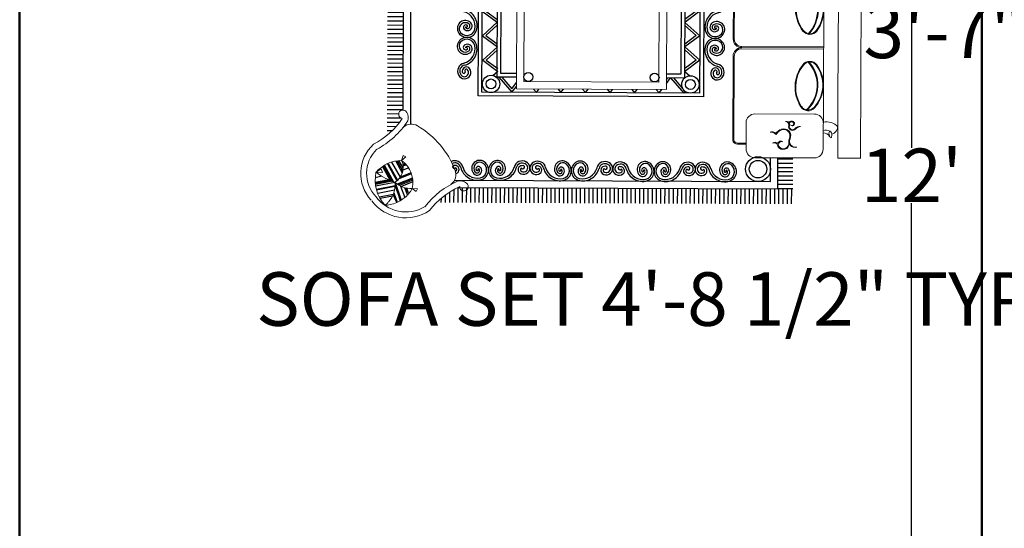
# Model space of a CAD drawing. Units: inches. Extents: x 147 to 1638, y 107 to 941.
# Tile 3 of 17: x 359 to 469, y 284 to 341. Entities that reach past the tile are written whole.
import ezdxf

# ---------------------------------------------------------------- set-up
doc = ezdxf.new("R2010")
doc.units = ezdxf.units.IN
doc.header["$MEASUREMENT"] = 0
for name, color, linetype, lineweight in [('A-ANNO-DIMS', 2, 'Continuous', 15), ('furniture', 50, 'Continuous', 18), ('wall', 7, 'Continuous', 60), ('walls', 7, 'Continuous', 50)]:
    doc.layers.add(name, color=color, linetype=linetype, lineweight=lineweight)
doc.layers.add('CARPET', color=40, linetype='Continuous')
doc.styles.get("Standard").update_dxf_attribs({"font": 'arial.ttf'})
doc.dimstyles.get("Standard").update_dxf_attribs({"dimtxt": 6, "dimasz": 3, "dimexe": 0.18, "dimexo": 0.0625, "dimgap": 0.09, "dimtad": 0, "dimtih": 1, "dimtoh": 1, "dimdec": 1, "dimzin": 0, "dimdsep": 46, "dimlunit": 3, "dimtxsty": 'Standard', "dimblk": 'ARCHTICK', "dimcen": 0.09, "dimadec": 0, "dimazin": 0, "dimtfac": 1, "dimtdec": 1, "dimtofl": 0, "dimtmove": 0, "dimatfit": 3, "dimfxl": 1, "dimtolj": 1, "dimtzin": 0, "dimarcsym": 0})

# ---------------------------------------------------------------- blocks, each defined once
blk = doc.blocks.new('_ArchTick')
at = {"color": 0, "linetype": 'ByBlock', "const_width": 0.15}
blk.add_lwpolyline([(-0.5, -0.5), (0.5, 0.5)], dxfattribs=at)
blk = doc.blocks.new('*D30')
at = {"layer": 'A-ANNO-DIMS', "color": 0, "lineweight": -2, "transparency": 16777216}
for p, q in [((460.3, 395.72), (458.86, 395.72)), ((459.04, 395.72), (459.04, 326.82)), ((459.04, 251.72), (459.04, 320.62)), ((460.3, 251.72), (458.86, 251.72))]:
    blk.add_line(p, q, dxfattribs=at)
at = {"layer": 'Defpoints', "color": 0, "lineweight": -2, "transparency": 16777216}
for p in [(460.36, 395.72), (459.04, 251.72), (460.36, 251.72)]:
    blk.add_point(p, dxfattribs=at)
at = {"layer": 'A-ANNO-DIMS', "color": 0, "lineweight": -2, "transparency": 16777216, "xscale": 3, "yscale": 3, "zscale": 3}
for p, rotation in [((459.04, 395.72), 90), ((459.04, 251.72), 270)]:
    blk.add_blockref('_ArchTick', p, dxfattribs=dict(at, rotation=rotation))
at = {"layer": 'A-ANNO-DIMS', "color": 0, "transparency": 16777216, "insert": (459.04, 323.72), "char_height": 6, "attachment_point": 5}
blk.add_mtext("\\A1;12'", dxfattribs=at)
blk = doc.blocks.new('X')
at = {"layer": 'furniture'}
for p, q in [((619.5149, -248.9209), (619.5149, -248.7654)), ((619.5149, -248.7654), (621.0036, -248.7654)), ((621.0036, -248.9205), (621.0036, -248.765)), ((619.5149, -248.9209), (619.7322, -248.9205)), ((619.7322, -248.9205), (620.6015, -248.9205)), ((621.0036, -248.9205), (620.6015, -248.9205)), ((619.5742, -249.0193), (619.752, -249.0193)), ((619.752, -249.0193), (620.6015, -249.0193)), ((620.2516, -249.5725), (620.2516, -249.0193)), ((620.259, -249.5725), (620.259, -249.0193)), ((620.259, -249.5725), (620.259, -249.0193)), ((620.2664, -249.5725), (620.2664, -249.0193)), ((620.9439, -249.0193), (620.6015, -249.0193)), ((619.5149, -249.0786), (619.5149, -249.4824)), ((619.8112, -249.4824), (619.8112, -249.0786)), ((620.7068, -249.4824), (620.7068, -249.0786)), ((621.0032, -249.4824), (621.0032, -249.0786)), ((619.5742, -249.5417), (619.752, -249.5417)), ((619.6049, -249.5417), (619.6049, -249.5987)), ((619.6124, -249.5417), (619.6124, -249.599)), ((620.9439, -249.5417), (620.7661, -249.5417)), ((620.9057, -249.5417), (620.9057, -249.599)), ((620.9131, -249.5417), (620.9131, -249.5987)), ((619.6334, -249.6243), (620.1998, -249.6243)), ((619.6334, -249.6317), (620.1998, -249.6317)), ((620.8846, -249.6243), (620.3183, -249.6243)), ((620.8846, -249.6317), (620.3183, -249.6317))]:
    blk.add_line(p, q, dxfattribs=at)
for centre, radius, start, end in [((619.7322, -248.9798), 0.0593, 90, 162.494), ((619.6556, -248.9979), 0.1044, 348.14652, 47.53007), ((620.8625, -248.9979), 0.1044, 132.46993, 191.85348), ((620.7859, -248.9798), 0.0593, 17.506, 90), ((619.635, -249.0188), 0.0496, 359.41182, 58.40348), ((619.6525, -249.0006), 0.0512, 338.60223, 29.59056), ((620.8656, -249.0006), 0.0512, 150.40944, 201.39777), ((620.8831, -249.0188), 0.0496, 121.59652, 180.58818), ((619.5742, -249.0786), 0.0593, 90, 180), ((619.752, -249.0786), 0.0593, 0, 90), ((620.007, -249.2904), 0.2333, 46.53167, 137.57273), ((620.007, -249.2476), 0.2283, 52.96969, 132.32477), ((620.007, -249.2476), 0.2234, 52.96969, 132.32477), ((620.5111, -249.2904), 0.2333, 42.42727, 133.46833), ((620.5111, -249.2476), 0.2283, 47.67523, 127.03031), ((620.5111, -249.2476), 0.2234, 47.67523, 127.03031), ((620.7661, -249.0786), 0.0593, 90, 180), ((620.9439, -249.0786), 0.0593, 0, 90), ((619.8932, -249.1226), 0.0593, 132.32477, 237.31292), ((620.007, -249.2904), 0.2283, 45.74065, 138.43075), ((619.8932, -249.1226), 0.0543, 132.32477, 237.31292), ((620.1088, -249.1127), 0.0543, 307.98154, 52.96969), ((620.1088, -249.1127), 0.0593, 307.98154, 52.96969), ((620.4092, -249.1127), 0.0593, 127.03031, 232.01846), ((620.5111, -249.2904), 0.2283, 41.56925, 134.25935), ((620.4092, -249.1127), 0.0543, 127.03031, 232.01846), ((620.6249, -249.1226), 0.0543, 302.68708, 47.67523), ((620.6249, -249.1226), 0.0593, 302.68708, 47.67523), ((619.6678, -249.1626), 0.0605, 312.99292, 349.19232), ((619.6905, -249.1804), 0.0373, 306.00619, 9.85592), ((619.994, -248.9656), 0.2459, 237.31292, 307.98154), ((619.994, -248.9656), 0.241, 237.31292, 307.98154), ((620.5241, -248.9656), 0.2459, 232.01846, 302.68708), ((620.5241, -248.9656), 0.241, 232.01846, 302.68708), ((620.8276, -249.1804), 0.0373, 170.14408, 233.99381), ((620.8503, -249.1626), 0.0605, 190.80768, 227.00708), ((619.6105, -249.2907), 0.0399, 81.34647, 244.80036), ((619.6138, -249.2892), 0.0378, 78.82007, 241.2356), ((619.6274, -249.2105), 0.0421, 161.95623, 295.85894), ((619.628, -249.2055), 0.0415, 168.85347, 291.99707), ((619.6641, -249.2863), 0.0471, 341.95623, 115.85894), ((619.6641, -249.2863), 0.0421, 341.95623, 115.85894), ((619.7278, -249.227), 0.0274, 132.99292, 265.5491), ((619.7278, -249.227), 0.0225, 132.99292, 262.0854), ((619.7361, -249.2716), 0.0251, 55.31815, 117.0875), ((619.7357, -249.2774), 0.0252, 3.68155, 113.53579), ((619.745, -249.2275), 0.014, 61.30612, 229.17278), ((619.7459, -249.2313), 0.0122, 73.4413, 214.10415), ((619.7406, -249.2356), 0.0182, 302.61304, 61.30612), ((619.7406, -249.2356), 0.0232, 306.28248, 61.30612), ((619.7361, -249.2716), 0.0251, 350.3606, 43.63947), ((620.7775, -249.2356), 0.0232, 118.69388, 233.71752), ((620.782, -249.2716), 0.0251, 136.36053, 189.6394), ((620.7824, -249.2774), 0.0252, 66.46421, 176.31845), ((620.7775, -249.2356), 0.0182, 118.69388, 237.38696), ((620.7731, -249.2275), 0.014, 310.82722, 118.69388), ((620.782, -249.2716), 0.0251, 62.9125, 124.68185), ((620.7722, -249.2313), 0.0122, 325.89585, 106.5587), ((620.7903, -249.227), 0.0274, 274.4509, 47.00708), ((620.7903, -249.227), 0.0225, 277.9146, 47.00708), ((620.854, -249.2863), 0.0471, 64.14106, 198.04377), ((620.854, -249.2863), 0.0421, 64.14106, 198.04377), ((620.8907, -249.2105), 0.0421, 244.14106, 18.04377), ((620.89, -249.2055), 0.0415, 248.00293, 11.14653), ((620.9043, -249.2892), 0.0378, 298.7644, 101.17993), ((620.9076, -249.2907), 0.0399, 295.19964, 98.65353), ((619.6028, -249.3007), 0.0227, 251.57956, 22.48814), ((619.6037, -249.3051), 0.024, 287.88795, 33.0148), ((619.6438, -249.2797), 0.0635, 295.85894, 341.95623), ((619.6438, -249.2797), 0.0684, 298.77648, 341.95623), ((620.8743, -249.2797), 0.0684, 198.04377, 241.22352), ((620.8743, -249.2797), 0.0635, 198.04377, 244.14106), ((620.9144, -249.3051), 0.024, 146.9852, 252.11205), ((620.9153, -249.3007), 0.0227, 157.51186, 288.42044), ((619.5921, -249.3513), 0.0246, 333.67342, 86.7751), ((619.5947, -249.3467), 0.0249, 321.27483, 48.99439), ((619.6335, -249.3751), 0.0539, 355.27866, 45.25264), ((619.6593, -249.3656), 0.0313, 333.5007, 56.06813), ((620.8588, -249.3656), 0.0313, 123.93187, 206.4993), ((620.8845, -249.3751), 0.0539, 134.74736, 184.72134), ((620.9233, -249.3467), 0.0249, 131.00561, 218.72517), ((620.926, -249.3513), 0.0246, 93.2249, 206.32658), ((619.5742, -249.4824), 0.0593, 180, 270), ((619.752, -249.4824), 0.0593, 270, 0), ((620.7661, -249.4824), 0.0593, 180, 270), ((620.9439, -249.4824), 0.0593, 270, 0), ((620.1998, -249.5725), 0.0593, 270, 0), ((620.1998, -249.5725), 0.0519, 270, 0), ((620.3183, -249.5725), 0.0593, 180, 270), ((620.3183, -249.5725), 0.0519, 180, 270), ((619.6387, -249.5984), 0.0338, 180.54468, 260.99104), ((619.6384, -249.5987), 0.0261, 179.37819, 258.97154), ((620.8796, -249.5987), 0.0261, 281.02846, 0.62181), ((620.8793, -249.5984), 0.0338, 279.00896, 359.45532)]:
    blk.add_arc(centre, radius, start, end, dxfattribs=at)
blk.add_ellipse((619.6743, -248.9709), major_axis=(-0.023, 0.0035), ratio=0.388107, start_param=3.141593, end_param=9.424778, dxfattribs=at)
at = {"layer": 'furniture', "extrusion": (0, 0, -1)}
blk.add_ellipse((620.8437, -248.9709), major_axis=(0.023, 0.0035), ratio=0.388107, start_param=3.141593, end_param=9.424778, dxfattribs=at)
blk = doc.blocks.new('sitting')
at = {"layer": 'CARPET'}
for p, q in [((0.3744, 0.8151), (0.3749, 0.9167)), ((0.403, 0.815), (0.4035, 0.9166)), ((0.4316, 0.8149), (0.432, 0.9165)), ((0.4602, 0.8148), (0.4606, 0.9164)), ((0.4887, 0.8147), (0.4892, 0.9163)), ((0.5173, 0.8145), (0.5178, 0.9161)), ((0.5459, 0.8144), (0.5463, 0.916)), ((0.5745, 0.8143), (0.5749, 0.9159)), ((0.603, 0.8142), (0.6035, 0.9158)), ((0.6316, 0.8141), (0.632, 0.9156)), ((0.6602, 0.8139), (0.6606, 0.9155)), ((0.6888, 0.8138), (0.6892, 0.9154)), ((2.1553, 0.8075), (2.1557, 0.9091)), ((2.1839, 0.8074), (2.1843, 0.909)), ((2.2125, 0.8073), (2.2129, 0.9089)), ((2.241, 0.8072), (2.2415, 0.9088)), ((2.2696, 0.8071), (2.27, 0.9087)), ((2.2982, 0.8069), (2.2986, 0.9085)), ((2.3268, 0.8068), (2.3272, 0.9084)), ((2.3553, 0.8067), (2.3558, 0.9083)), ((2.4602, 0.8713), (2.3589, 0.8717)), ((2.4603, 0.8998), (2.359, 0.9003)), ((0.3793, 0.8151), (0.3774, 0.3798)), ((0.6912, 0.81), (0.3793, 0.8151)), ((0.4301, 0.8149), (0.4301, 0.8143)), ((2.3583, 0.8067), (2.1476, 0.8076)), ((2.349, -1.3602), (2.3583, 0.8067)), ((2.4599, 0.8141), (2.3586, 0.8145)), ((2.46, 0.8427), (2.3588, 0.8431)), ((0.3789, 0.7373), (0.2773, 0.7377)), ((0.379, 0.7658), (0.2774, 0.7663)), ((0.3791, 0.7944), (0.2775, 0.7949)), ((0.3791, 0.7643), (0.3785, 0.7643)), ((0.4299, 0.7635), (0.4282, 0.3764)), ((0.6904, 0.7592), (0.4299, 0.7635)), ((2.3073, 0.7561), (2.1474, 0.7568)), ((2.2981, -1.3815), (2.3073, 0.7561)), ((2.4597, 0.757), (2.3584, 0.7574)), ((2.4598, 0.7855), (2.3585, 0.786)), ((0.3786, 0.6801), (0.277, 0.6806)), ((0.3788, 0.7087), (0.2772, 0.7091)), ((2.4593, 0.6712), (2.358, 0.6717)), ((2.4594, 0.6998), (2.3582, 0.7002)), ((2.4596, 0.7284), (2.3583, 0.7288)), ((0.3784, 0.623), (0.2768, 0.6234)), ((0.3785, 0.6515), (0.2769, 0.652)), ((2.4591, 0.6141), (2.3578, 0.6145)), ((2.4592, 0.6427), (2.3579, 0.6431)), ((0.378, 0.5372), (0.2764, 0.5377)), ((0.3782, 0.5658), (0.2766, 0.5663)), ((0.3783, 0.5944), (0.2767, 0.5948)), ((2.4588, 0.5569), (2.3576, 0.5574)), ((2.4589, 0.5855), (2.3577, 0.586)), ((0.3778, 0.4801), (0.2762, 0.4805)), ((0.3779, 0.5087), (0.2763, 0.5091)), ((2.4585, 0.4712), (2.3572, 0.4717)), ((2.4586, 0.4998), (2.3573, 0.5002)), ((2.4587, 0.5284), (2.3574, 0.5288)), ((0.3775, 0.4229), (0.2759, 0.4234)), ((0.3777, 0.4515), (0.2761, 0.452)), ((2.4582, 0.4141), (2.3569, 0.4145)), ((2.4583, 0.4426), (2.3571, 0.4431)), ((0.3774, 0.3944), (0.2758, 0.3948)), ((2.458, 0.3569), (2.3567, 0.3574)), ((2.4581, 0.3855), (2.3568, 0.3859)), ((1.065, 0.178), (1.1552, 0.2792)), ((1.1552, 0.2792), (1.2313, 0.1773)), ((1.2313, 0.1773), (1.3215, 0.2785)), ((1.3215, 0.2785), (1.3976, 0.1766)), ((1.3976, 0.1766), (1.4877, 0.2778)), ((1.4877, 0.2778), (1.5638, 0.1759)), ((2.4576, 0.2712), (2.3563, 0.2716)), ((2.4577, 0.2998), (2.3565, 0.3002)), ((2.4578, 0.3283), (2.3566, 0.3288)), ((1.0854, 0.1779), (1.1542, 0.2552)), ((1.1542, 0.2552), (1.2122, 0.1774)), ((1.2516, 0.1772), (1.3204, 0.2544)), ((1.3204, 0.2544), (1.3785, 0.1767)), ((1.4179, 0.1765), (1.4867, 0.2537)), ((1.4867, 0.2537), (1.5447, 0.176)), ((1.5638, 0.1759), (1.5928, 0.2111)), ((2.4574, 0.214), (2.3561, 0.2145)), ((2.4575, 0.2426), (2.3562, 0.2431)), ((1.0646, 0.0827), (0.9634, 0.1728)), ((1.0647, 0.103), (0.9951, 0.165)), ((1.6077, 0.0803), (1.7096, 0.1696)), ((1.6077, 0.1007), (1.6779, 0.1621)), ((1.7096, 0.1696), (1.6979, 0.1786)), ((2.4571, 0.1569), (2.3558, 0.1573)), ((2.4572, 0.1855), (2.356, 0.1859)), ((0.9627, 0.0066), (1.0646, 0.0827)), ((1.6441, 0.0527), (1.6077, 0.0803)), ((2.4567, 0.0712), (2.3555, 0.0716)), ((2.4569, 0.0997), (2.3556, 0.1002)), ((2.457, 0.1283), (2.3557, 0.1288)), ((1.0444, -0.0662), (0.9627, 0.0066)), ((0.9868, 0.0055), (1.0646, 0.0636)), ((1.0444, -0.0458), (0.9868, 0.0055)), ((1.6188, 0.0528), (1.6076, 0.0613)), ((1.6859, -0.0168), (1.7089, 0.0034)), ((1.7089, 0.0034), (1.6861, 0.0207)), ((2.4565, 0.014), (2.3552, 0.0145)), ((2.4566, 0.0426), (2.3554, 0.043)), ((2.4563, -0.0431), (2.355, -0.0427)), ((2.4564, -0.0146), (2.3551, -0.0141)), ((0.962, -0.1597), (1.0442, -0.0983)), ((0.9861, -0.1607), (1.0441, -0.1174)), ((2.4559, -0.1288), (2.3546, -0.1284)), ((2.456, -0.1003), (2.3547, -0.0998)), ((2.4561, -0.0717), (2.3549, -0.0713)), ((1.0436, -0.2324), (0.962, -0.1597)), ((1.0437, -0.2121), (0.9861, -0.1607)), ((1.6852, -0.183), (1.7082, -0.1629)), ((1.7082, -0.1629), (1.6854, -0.1455)), ((2.4557, -0.186), (2.3544, -0.1856)), ((2.4558, -0.1574), (2.3545, -0.157)), ((0.9613, -0.326), (1.0435, -0.2646)), ((2.4554, -0.2431), (2.3541, -0.2427)), ((2.4555, -0.2146), (2.3543, -0.2141)), ((1.0429, -0.3987), (0.9613, -0.326)), ((0.9854, -0.327), (1.0434, -0.2837)), ((1.043, -0.3784), (0.9854, -0.327)), ((1.6845, -0.3493), (1.7075, -0.3291)), ((1.7075, -0.3291), (1.6847, -0.3118)), ((2.455, -0.3289), (2.3538, -0.3284)), ((2.4552, -0.3003), (2.3539, -0.2999)), ((2.4553, -0.2717), (2.354, -0.2713)), ((0.3734, -0.5318), (0.374, -0.383)), ((0.4242, -0.5353), (0.4248, -0.38)), ((2.4548, -0.386), (2.3535, -0.3856)), ((2.4549, -0.3574), (2.3537, -0.357)), ((0.9606, -0.4922), (1.0428, -0.4308)), ((0.9847, -0.4933), (1.0427, -0.4499)), ((2.4546, -0.4432), (2.3533, -0.4427)), ((2.4547, -0.4146), (2.3534, -0.4142)), ((1.0422, -0.5649), (0.9606, -0.4922)), ((1.0423, -0.5446), (0.9847, -0.4933)), ((1.6838, -0.5155), (1.7068, -0.4954)), ((1.7068, -0.4954), (1.684, -0.478)), ((2.4542, -0.5289), (2.3529, -0.5285)), ((2.4543, -0.5003), (2.353, -0.4999)), ((2.4544, -0.4717), (2.3532, -0.4713)), ((0.9599, -0.6585), (1.0421, -0.5971)), ((2.4539, -0.586), (2.3527, -0.5856)), ((2.4541, -0.5575), (2.3528, -0.557)), ((1.0415, -0.7312), (0.9599, -0.6585)), ((0.984, -0.6595), (1.042, -0.6162)), ((1.0416, -0.7109), (0.984, -0.6595)), ((1.6831, -0.6818), (1.7061, -0.6617)), ((1.7061, -0.6617), (1.6833, -0.6443)), ((2.4537, -0.6432), (2.3524, -0.6428)), ((2.4538, -0.6146), (2.3526, -0.6142)), ((2.4533, -0.7289), (2.3521, -0.7285)), ((2.4535, -0.7003), (2.3522, -0.6999)), ((2.4536, -0.6718), (2.3523, -0.6713)), ((0.9592, -0.8247), (1.0414, -0.7634)), ((0.9832, -0.8258), (1.0413, -0.7824)), ((2.4531, -0.7861), (2.3518, -0.7856)), ((2.4532, -0.7575), (2.3519, -0.7571)), ((1.0408, -0.8975), (0.9592, -0.8247)), ((1.0409, -0.8771), (0.9832, -0.8258)), ((1.6824, -0.8481), (1.7054, -0.8279)), ((1.7054, -0.8279), (1.6825, -0.8106)), ((2.4528, -0.8432), (2.3516, -0.8428)), ((2.453, -0.8146), (2.3517, -0.8142)), ((0.9585, -0.991), (1.0407, -0.9296)), ((2.4525, -0.9289), (2.3512, -0.9285)), ((2.4526, -0.9004), (2.3513, -0.8999)), ((2.4527, -0.8718), (2.3515, -0.8714)), ((1.0597, -1.0812), (0.9585, -0.991)), ((0.9825, -0.992), (1.0406, -0.9487)), ((1.0598, -1.0608), (0.9825, -0.992)), ((1.6027, -1.0835), (1.7047, -0.9942)), ((1.6028, -1.0632), (1.6806, -0.995)), ((1.6806, -0.995), (1.6392, -0.9636)), ((1.7047, -0.9942), (1.6645, -0.9637)), ((2.4522, -0.9861), (2.351, -0.9857)), ((2.4524, -0.9575), (2.3511, -0.9571)), ((2.452, -1.0432), (2.3507, -1.0428)), ((2.4521, -1.0147), (2.3508, -1.0142)), ((1.0645, -1.0959), (1.1557, -1.1962)), ((1.0848, -1.0956), (1.1544, -1.1721)), ((1.1544, -1.1721), (1.2117, -1.0938)), ((1.1557, -1.1962), (1.2307, -1.0935)), ((1.2307, -1.0935), (1.3219, -1.1938)), ((1.2511, -1.0932), (1.3206, -1.1697)), ((1.3206, -1.1697), (1.3779, -1.0914)), ((1.3219, -1.1938), (1.397, -1.0911)), ((1.397, -1.0911), (1.4882, -1.1914)), ((1.4173, -1.0908), (1.4869, -1.1674)), ((1.4869, -1.1674), (1.5442, -1.089)), ((1.4882, -1.1914), (1.5632, -1.0887)), ((1.5632, -1.0887), (1.5926, -1.1237)), ((2.4516, -1.129), (2.3504, -1.1285)), ((2.4517, -1.1004), (2.3505, -1.1)), ((2.4519, -1.0718), (2.3506, -1.0714)), ((2.4514, -1.1861), (2.3501, -1.1857)), ((2.4515, -1.1575), (2.3502, -1.1571)), ((2.4511, -1.2433), (2.3499, -1.2428)), ((2.4513, -1.2147), (2.35, -1.2143)), ((0.3701, -1.3201), (0.2685, -1.3197)), ((0.3458, -1.2914), (0.2686, -1.2911)), ((0.3684, -1.73), (0.3702, -1.2947)), ((0.4194, -1.6792), (0.421, -1.2917)), ((2.4508, -1.329), (2.3495, -1.3286)), ((2.4509, -1.3004), (2.3496, -1.3)), ((2.451, -1.2718), (2.3498, -1.2714)), ((0.3699, -1.3773), (0.2683, -1.3768)), ((0.37, -1.3487), (0.2684, -1.3483)), ((2.4507, -1.3576), (2.3494, -1.3571)), ((2.4505, -1.3861), (2.3623, -1.3858)), ((0.3695, -1.463), (0.2679, -1.4626)), ((0.3696, -1.4344), (0.268, -1.434)), ((0.3697, -1.4058), (0.2681, -1.4054)), ((2.4504, -1.4147), (2.3793, -1.4144)), ((2.4503, -1.4433), (2.3989, -1.4431)), ((0.3693, -1.5201), (0.2677, -1.5197)), ((0.3694, -1.4916), (0.2678, -1.4911)), ((2.4502, -1.4719), (2.4215, -1.4717)), ((0.369, -1.5773), (0.2674, -1.5769)), ((0.3691, -1.5487), (0.2675, -1.5483)), ((0.3686, -1.663), (0.267, -1.6626)), ((0.3688, -1.6344), (0.2672, -1.634)), ((0.3689, -1.6059), (0.2673, -1.6054)), ((2.2845, -1.6663), (2.3262, -1.7708)), ((2.2896, -1.6655), (2.3296, -1.7657)), ((2.2995, -1.6644), (2.3358, -1.7553)), ((2.3112, -1.6637), (2.3424, -1.7417)), ((0.3684, -1.7202), (0.2668, -1.7197)), ((0.3685, -1.6916), (0.2669, -1.6912)), ((0.3684, -1.73), (1.8242, -1.7316)), ((0.3685, -1.6792), (0.3686, -1.6792)), ((0.3917, -1.8317), (0.3922, -1.7301)), ((0.4194, -1.6792), (1.9199, -1.6809)), ((0.4203, -1.8318), (0.4207, -1.7302)), ((0.4489, -1.8319), (0.4493, -1.7303)), ((0.4775, -1.832), (0.4779, -1.7304)), ((0.506, -1.8322), (0.5065, -1.7306)), ((0.5346, -1.8323), (0.535, -1.7307)), ((0.5632, -1.8324), (0.5636, -1.7308)), ((0.5917, -1.8325), (0.5922, -1.7309)), ((0.6203, -1.8327), (0.6208, -1.7311)), ((0.6489, -1.8328), (0.6493, -1.7312)), ((0.6775, -1.8329), (0.6779, -1.7313)), ((0.6775, -1.8329), (0.6779, -1.7313)), ((0.706, -1.833), (0.7065, -1.7314)), ((0.7346, -1.8331), (0.7351, -1.7315)), ((0.7632, -1.8333), (0.7636, -1.7317)), ((0.7918, -1.8334), (0.7922, -1.7318)), ((0.8203, -1.8335), (0.8208, -1.7319)), ((0.8489, -1.8336), (0.8494, -1.732)), ((0.8775, -1.8338), (0.8779, -1.7322)), ((0.9061, -1.8339), (0.9065, -1.7323)), ((0.9346, -1.834), (0.9351, -1.7324)), ((0.9632, -1.8341), (0.9637, -1.7325)), ((0.9632, -1.8341), (0.9637, -1.7325)), ((0.9918, -1.8342), (0.9922, -1.7326)), ((1.0204, -1.8344), (1.0208, -1.7328)), ((1.0489, -1.8345), (1.0494, -1.7329)), ((1.0775, -1.8346), (1.078, -1.733)), ((1.1061, -1.8347), (1.1065, -1.7331)), ((1.1347, -1.8349), (1.1351, -1.7333)), ((2.1669, -1.7607), (2.2209, -1.7306)), ((2.1682, -1.7716), (2.2377, -1.7329)), ((2.1869, -1.7158), (2.1934, -1.732)), ((2.1905, -1.7124), (2.1981, -1.7313)), ((2.1949, -1.7086), (2.2037, -1.7307)), ((2.2165, -1.6925), (2.2322, -1.7319)), ((2.2497, -1.6758), (2.2797, -1.7508)), ((2.2561, -1.6735), (2.2901, -1.7588)), ((2.3392, -1.7487), (2.4162, -1.7184)), ((2.3496, -1.7218), (2.4007, -1.7017)), ((2.3514, -1.7152), (2.3825, -1.7029)), ((2.353, -1.7075), (2.3836, -1.6955)), ((1.1632, -1.835), (1.1637, -1.7334)), ((1.1918, -1.8351), (1.1923, -1.7335)), ((1.2204, -1.8352), (1.2208, -1.7336)), ((1.249, -1.8353), (1.2494, -1.7337)), ((1.249, -1.8353), (1.2494, -1.7337)), ((1.2775, -1.8355), (1.278, -1.7339)), ((1.3061, -1.8356), (1.3066, -1.734)), ((1.3347, -1.8357), (1.3351, -1.7341)), ((1.3633, -1.8358), (1.3637, -1.7342)), ((1.3918, -1.8359), (1.3923, -1.7344)), ((1.4204, -1.8361), (1.4209, -1.7345)), ((1.449, -1.8362), (1.4494, -1.7346)), ((1.4776, -1.8363), (1.478, -1.7347)), ((1.5061, -1.8364), (1.5066, -1.7348)), ((1.5347, -1.8366), (1.5351, -1.735)), ((1.5347, -1.8366), (1.5351, -1.735)), ((1.5633, -1.8367), (1.5637, -1.7351)), ((1.5919, -1.8368), (1.5923, -1.7352)), ((1.6204, -1.8369), (1.6209, -1.7353)), ((1.649, -1.837), (1.6494, -1.7354)), ((1.6776, -1.8372), (1.678, -1.7356)), ((1.7062, -1.8373), (1.7066, -1.7357)), ((1.7347, -1.8374), (1.7352, -1.7358)), ((1.7633, -1.8375), (1.7637, -1.7359)), ((1.7919, -1.8377), (1.7923, -1.7361)), ((1.8205, -1.8378), (1.8209, -1.7362)), ((1.8205, -1.8378), (1.8209, -1.7362)), ((1.849, -1.8379), (1.8494, -1.7604)), ((1.8776, -1.838), (1.878, -1.7463)), ((1.9062, -1.8381), (1.9065, -1.7539)), ((1.9348, -1.8383), (1.935, -1.7772)), ((1.9348, -1.8383), (1.935, -1.7772)), ((2.1696, -1.7798), (2.2486, -1.7358)), ((2.1767, -1.8083), (2.2798, -1.7509)), ((2.1854, -1.8315), (2.2996, -1.7679)), ((2.1876, -1.8364), (2.3032, -1.7719)), ((2.1988, -1.8576), (2.3106, -1.7953)), ((2.3142, -1.7864), (2.3404, -1.9165)), ((2.3154, -1.7846), (2.4341, -1.7427)), ((2.3177, -1.7875), (2.4393, -1.7513)), ((2.3375, -1.7853), (2.3628, -1.9109)), ((2.3403, -1.7854), (2.3836, -1.7684)), ((2.3425, -1.7855), (2.3676, -1.9096)), ((2.3667, -1.7885), (2.3896, -1.9022)), ((2.3849, -1.7941), (2.4485, -1.7704)), ((2.3952, -1.797), (2.4141, -1.8911)), ((2.3975, -1.7979), (2.448, -1.7755)), ((1.9633, -1.8384), (1.9635, -1.8042)), ((2.2023, -1.8633), (2.3072, -1.8049)), ((2.2069, -1.8702), (2.3018, -1.8173)), ((2.297, -1.8281), (2.3153, -1.9188)), ((2.3011, -1.8189), (2.3211, -1.9184)), ((2.3067, -1.8053), (2.3293, -1.9175)), ((2.4068, -1.802), (2.4237, -1.8859)), ((2.2731, -1.8735), (2.2823, -1.919))]:
    blk.add_line(p, q, dxfattribs=at)
for points in [[(0.9321, -1.2188), (0.9386, 0.3056), (1.7356, 0.3022), (1.7291, -1.2222)], [(0.9576, -1.1935), (0.9639, 0.2801), (1.7101, 0.2769), (1.7038, -1.1967)]]:
    blk.add_lwpolyline(points, close=True, dxfattribs=at)
for points in [[(1.0645, 0.0551), (1.065, 0.178), (1.6081, 0.1757), (1.6075, 0.0528)], [(1.0899, 0.055), (1.0903, 0.1525), (1.5826, 0.1504), (1.5821, 0.0529)], [(1.6032, -0.9634), (1.6026, -1.0947), (1.0596, -1.0923), (1.0602, -0.9611)], [(1.5778, -0.9633), (1.5774, -1.0692), (1.0851, -1.0671), (1.0856, -0.9612)]]:
    blk.add_lwpolyline(points, dxfattribs=at)
for centre, radius in [((0.5147, 0.6796), 0.0843), ((0.5147, 0.6796), 0.0589), ((2.2246, 0.6725), 0.0843), ((2.2246, 0.6725), 0.0589), ((1.022, 0.2174), 0.0589), ((1.6516, 0.2147), 0.0589), ((1.022, 0.2174), 0.0335), ((1.6516, 0.2147), 0.0335), ((1.1262, -0.0259), 0.0301), ((1.6047, -0.028), 0.0301), ((1.1225, -0.881), 0.0301), ((1.601, -0.883), 0.0301), ((1.0184, -1.1325), 0.0589), ((1.0184, -1.1325), 0.0335), ((1.6479, -1.1352), 0.0589), ((1.6479, -1.1352), 0.0335), ((0.505, -1.5948), 0.0843), ((0.505, -1.5948), 0.0589)]:
    blk.add_circle(centre, radius, dxfattribs=at)
for centre, radius, start, end in [((0.497, 0.4669), 0.067, 33.92326, 162.74749), ((0.5416, 0.4551), 0.1132, 163.72753, 224.16333), ((0.5428, 0.4571), 0.1008, 166.99629, 238.96019), ((0.4977, 0.4665), 0.0548, 20.90664, 165.92882), ((0.4936, 0.4564), 0.0315, 41.04313, 239.89648), ((0.4936, 0.4564), 0.0169, 41.04313, 239.89648), ((0.5086, 0.4733), 0.0538, 235.07981, 35.18035), ((0.5086, 0.4759), 0.0415, 235.36127, 14.07703), ((0.5048, 0.4662), 0.0166, 231.08782, 41.04313), ((0.5048, 0.4662), 0.00198, 231.08782, 41.04313), ((2.2298, 0.466), 0.0538, 144.33076, 304.4313), ((2.2413, 0.4595), 0.067, 16.76363, 145.58785), ((2.2297, 0.4686), 0.0415, 165.43408, 304.14985), ((2.2406, 0.459), 0.0548, 13.58229, 158.60447), ((2.2335, 0.4588), 0.0166, 138.46799, 308.4233), ((2.1954, 0.45), 0.1008, 284.1961, 12.51483), ((2.2447, 0.449), 0.0315, 299.61464, 138.46799), ((2.1966, 0.448), 0.1132, 284.45049, 15.78359), ((0.5005, 0.4578), 0.00755, 65.8585, 269.29351), ((1.1039, 0.3982), 0.0436, 112.88129, 307.21618), ((1.1031, 0.3985), 0.0284, 110.32478, 311.53076), ((1.1129, 0.3899), 0.055, 11.99051, 119.18067), ((1.1129, 0.3899), 0.0404, 11.99051, 119.18067), ((1.1077, 0.403), 0.011, 65.50738, 327.11735), ((1.1131, 0.3853), 0.0277, 308.26022, 91.73038), ((1.264, 0.4277), 0.1008, 194.1961, 282.51483), ((1.2799, 0.3933), 0.0538, 54.33076, 214.4313), ((1.2629, 0.3785), 0.0315, 209.61464, 48.46799), ((1.2825, 0.3934), 0.0415, 75.43408, 214.14985), ((1.2728, 0.3896), 0.0166, 48.46799, 218.4233), ((1.273, 0.3825), 0.0548, 283.58229, 68.60447), ((1.2734, 0.3818), 0.067, 286.76363, 55.58785), ((1.4074, 0.3811), 0.067, 123.92326, 252.74749), ((1.4078, 0.3819), 0.0548, 110.90664, 255.92882), ((1.401, 0.3927), 0.0538, 325.07981, 125.18035), ((1.4179, 0.3777), 0.0315, 131.04313, 329.89648), ((1.3984, 0.3928), 0.0415, 325.36127, 104.07703), ((1.4172, 0.4269), 0.1008, 256.99629, 345.31502), ((1.4081, 0.389), 0.0166, 321.08782, 131.04313), ((1.5679, 0.3879), 0.055, 60.33045, 167.52061), ((1.5679, 0.3879), 0.0404, 60.33045, 167.52061), ((1.5677, 0.3833), 0.0277, 87.78073, 231.2509), ((1.577, 0.3961), 0.0436, 232.29494, 66.62983), ((1.5778, 0.3964), 0.0284, 227.98036, 69.18634), ((1.5733, 0.4009), 0.011, 212.39376, 114.00374), ((2.2335, 0.4588), 0.00198, 138.46799, 308.4233), ((2.2447, 0.449), 0.0169, 299.61464, 138.46799), ((2.2377, 0.4504), 0.00755, 270.2176, 113.65261), ((1.1133, 0.3856), 0.012, 316.00944, 72.44807), ((1.262, 0.4266), 0.1132, 194.45049, 285.78359), ((1.2629, 0.3785), 0.0169, 209.61464, 48.46799), ((1.2643, 0.3854), 0.00755, 180.2176, 23.65261), ((1.2728, 0.3896), 0.00198, 48.46799, 218.4233), ((1.4192, 0.4258), 0.1132, 253.72753, 345.06062), ((1.4179, 0.3777), 0.0169, 131.04313, 329.89648), ((1.4081, 0.389), 0.00198, 321.08782, 131.04313), ((1.4165, 0.3846), 0.00755, 155.8585, 359.29351), ((1.5675, 0.3835), 0.012, 107.06305, 223.50168), ((2.2332, 0.299), 0.055, 101.99051, 209.18067), ((2.2332, 0.299), 0.0404, 101.99051, 209.18067), ((2.2249, 0.29), 0.0436, 202.88129, 37.21618), ((2.2246, 0.2892), 0.0284, 200.32478, 41.53076), ((2.2201, 0.2937), 0.011, 155.50738, 57.11735), ((2.2378, 0.2991), 0.0277, 38.26022, 181.73038), ((2.2376, 0.2994), 0.012, 46.00944, 162.44807), ((2.2327, 0.1959), 0.055, 150.33045, 257.52061), ((2.2245, 0.205), 0.0436, 322.29494, 156.62983), ((2.2327, 0.1959), 0.0404, 150.33045, 257.52061), ((2.2243, 0.2058), 0.0284, 317.98036, 159.18634), ((2.2197, 0.2012), 0.011, 302.39376, 204.00374), ((2.2374, 0.1957), 0.0277, 177.78073, 321.2509), ((2.1937, 0.0451), 0.1008, 346.99629, 75.31502), ((2.1948, 0.0472), 0.1132, 343.72753, 75.06062), ((2.2371, 0.1955), 0.012, 197.06305, 313.50168), ((2.2279, 0.0289), 0.0538, 55.07981, 215.18035), ((2.2278, 0.0263), 0.0415, 55.36127, 194.07703), ((2.2429, 0.0458), 0.0315, 221.04313, 59.89648), ((2.2395, 0.0353), 0.067, 213.92326, 342.74749), ((2.2388, 0.0358), 0.0548, 200.90664, 345.92882), ((2.2317, 0.036), 0.0166, 51.08782, 221.04313), ((2.2317, 0.036), 0.00198, 51.08782, 221.04313), ((2.2429, 0.0458), 0.0169, 221.04313, 59.89648), ((2.236, 0.0445), 0.00755, 245.8585, 89.29351), ((2.2275, -0.0922), 0.0538, 144.33076, 304.4313), ((2.239, -0.0986), 0.067, 16.76363, 145.58785), ((2.2383, -0.0991), 0.0548, 13.58229, 158.60447), ((2.2274, -0.0895), 0.0415, 165.43408, 304.14985), ((2.2312, -0.0993), 0.0166, 138.46799, 308.4233), ((2.1931, -0.1081), 0.1008, 284.1961, 12.51483), ((2.2424, -0.1091), 0.0315, 299.61464, 138.46799), ((2.1942, -0.1101), 0.1132, 284.45049, 15.78359), ((2.2312, -0.0993), 0.00198, 138.46799, 308.4233), ((2.2424, -0.1091), 0.0169, 299.61464, 138.46799), ((2.2354, -0.1077), 0.00755, 270.2176, 113.65261), ((2.2309, -0.2591), 0.055, 101.99051, 209.18067), ((2.2226, -0.2681), 0.0436, 202.88129, 37.21618), ((2.2309, -0.2591), 0.0404, 101.99051, 209.18067), ((2.2223, -0.2689), 0.0284, 200.32478, 41.53076), ((2.2178, -0.2644), 0.011, 155.50738, 57.11735), ((2.2355, -0.259), 0.0277, 38.26022, 181.73038), ((2.2352, -0.2587), 0.012, 46.00944, 162.44807), ((2.22, -0.3553), 0.0436, 322.29494, 156.62983), ((2.2197, -0.3545), 0.0284, 317.98036, 159.18634), ((2.2282, -0.3643), 0.055, 150.33045, 257.52061), ((2.2282, -0.3643), 0.0404, 150.33045, 257.52061), ((2.2152, -0.359), 0.011, 302.39376, 204.00374), ((2.2328, -0.3646), 0.0277, 177.78073, 321.2509), ((2.2326, -0.3648), 0.012, 197.06305, 313.50168), ((2.1892, -0.5151), 0.1008, 346.99629, 75.31502), ((2.1903, -0.5131), 0.1132, 343.72753, 75.06062), ((2.2234, -0.5313), 0.0538, 55.07981, 215.18035), ((2.2233, -0.5339), 0.0415, 55.36127, 194.07703), ((2.2276, -0.5255), 0.0166, 51.08782, 221.04313), ((2.2384, -0.5144), 0.0315, 221.04313, 59.89648), ((2.2384, -0.5144), 0.0169, 221.04313, 59.89648), ((2.2276, -0.5255), 0.00198, 51.08782, 221.04313), ((2.232, -0.5171), 0.00755, 245.8585, 89.29351), ((2.2345, -0.6588), 0.067, 16.76363, 145.58785), ((2.235, -0.5249), 0.067, 213.92326, 342.74749), ((2.2342, -0.5244), 0.0548, 200.90664, 345.92882), ((2.2229, -0.6524), 0.0538, 144.33076, 304.4313), ((2.2229, -0.6498), 0.0415, 165.43408, 304.14985), ((2.2337, -0.6593), 0.0548, 13.58229, 158.60447), ((2.2271, -0.6608), 0.0166, 138.46799, 308.4233), ((2.1886, -0.6683), 0.1008, 284.1961, 12.51483), ((2.2378, -0.6694), 0.0315, 299.61464, 138.46799), ((2.1897, -0.6703), 0.1132, 284.45049, 15.78359), ((2.2378, -0.6694), 0.0169, 299.61464, 138.46799), ((2.2271, -0.6608), 0.00198, 138.46799, 308.4233), ((2.2314, -0.6693), 0.00755, 270.2176, 113.65261), ((2.2263, -0.8194), 0.055, 101.99051, 209.18067), ((2.2263, -0.8194), 0.0404, 101.99051, 209.18067), ((2.2309, -0.8192), 0.0277, 38.26022, 181.73038), ((2.218, -0.8284), 0.0436, 202.88129, 37.21618), ((2.2177, -0.8292), 0.0284, 200.32478, 41.53076), ((2.2132, -0.8246), 0.011, 155.50738, 57.11735), ((2.2307, -0.819), 0.012, 46.00944, 162.44807), ((2.2242, -0.9246), 0.055, 150.33045, 257.52061), ((2.216, -0.9155), 0.0436, 322.29494, 156.62983), ((2.2242, -0.9246), 0.0404, 150.33045, 257.52061), ((2.2157, -0.9147), 0.0284, 317.98036, 159.18634), ((2.2112, -0.9192), 0.011, 302.39376, 204.00374), ((2.2288, -0.9248), 0.0277, 177.78073, 321.2509), ((2.2286, -0.925), 0.012, 197.06305, 313.50168), ((2.1852, -1.0753), 0.1008, 346.99629, 75.31502), ((2.1863, -1.0733), 0.1132, 343.72753, 75.06062), ((2.2194, -1.0915), 0.0538, 55.07981, 215.18035), ((2.2193, -1.0941), 0.0415, 55.36127, 194.07703), ((2.2344, -1.0746), 0.0315, 221.04313, 59.89648), ((2.2344, -1.0746), 0.0169, 221.04313, 59.89648), ((2.231, -1.0852), 0.067, 213.92326, 342.74749), ((2.2302, -1.0847), 0.0548, 200.90664, 345.92882), ((2.2231, -1.0844), 0.0166, 51.08782, 221.04313), ((2.2231, -1.0844), 0.00198, 51.08782, 221.04313), ((2.2275, -1.076), 0.00755, 245.8585, 89.29351), ((2.2189, -1.2126), 0.0538, 144.33076, 304.4313), ((2.2305, -1.2191), 0.067, 16.76363, 145.58785), ((2.2189, -1.21), 0.0415, 165.43408, 304.14985), ((2.2297, -1.2195), 0.0548, 13.58229, 158.60447), ((2.2338, -1.2296), 0.0315, 299.61464, 138.46799), ((2.1857, -1.2305), 0.1132, 284.45049, 15.78359), ((1.2544, -1.3426), 0.1132, 73.72753, 165.06062), ((1.2564, -1.3437), 0.1008, 76.99629, 165.31502), ((1.2558, -1.2945), 0.0315, 311.04313, 149.89648), ((1.2658, -1.2986), 0.0548, 290.90664, 75.92882), ((1.2663, -1.2979), 0.067, 303.92326, 72.74749), ((1.4002, -1.2984), 0.067, 106.76363, 235.58785), ((1.4007, -1.2991), 0.0548, 103.58229, 248.60447), ((1.4107, -1.295), 0.0315, 29.61464, 228.46799), ((1.4117, -1.3432), 0.1132, 14.45049, 105.78359), ((1.4096, -1.3443), 0.1008, 14.1961, 102.51483), ((2.2231, -1.221), 0.0166, 138.46799, 308.4233), ((2.1846, -1.2285), 0.1008, 284.1961, 12.51483), ((2.2338, -1.2296), 0.0169, 299.61464, 138.46799), ((2.2231, -1.221), 0.00198, 138.46799, 308.4233), ((2.2274, -1.2295), 0.00755, 270.2176, 113.65261), ((0.5381, -1.2235), 0.1132, 217.11392, 255.06062), ((0.5393, -1.2215), 0.1008, 221.67675, 255.31502), ((0.5002, -1.3723), 0.0404, 330.33045, 77.52061), ((0.5002, -1.3723), 0.055, 330.33045, 77.52061), ((1.0966, -1.3129), 0.0436, 52.29494, 246.62983), ((1.0958, -1.3131), 0.0284, 47.98036, 249.18634), ((1.1057, -1.3047), 0.055, 240.33045, 347.52061), ((1.1057, -1.3047), 0.0404, 240.33045, 347.52061), ((1.1003, -1.3177), 0.011, 32.39376, 294.00374), ((1.1059, -1.3), 0.0277, 267.78073, 51.2509), ((1.1061, -1.3003), 0.012, 287.06305, 43.50168), ((1.2726, -1.3095), 0.0538, 145.07981, 305.18035), ((1.2753, -1.3096), 0.0415, 145.36127, 284.07703), ((1.2558, -1.2945), 0.0169, 311.04313, 149.89648), ((1.2656, -1.3057), 0.0166, 141.08782, 311.04313), ((1.2571, -1.3014), 0.00755, 335.8585, 179.29351), ((1.2656, -1.3057), 0.00198, 141.08782, 311.04313), ((1.3937, -1.3099), 0.0538, 234.33076, 34.4313), ((1.3911, -1.31), 0.0415, 255.43408, 34.14985), ((1.4008, -1.3062), 0.0166, 228.46799, 38.4233), ((1.4107, -1.295), 0.0169, 29.61464, 228.46799), ((1.4008, -1.3062), 0.00198, 228.46799, 38.4233), ((1.4093, -1.302), 0.00755, 0.2176, 203.65261), ((1.5607, -1.3065), 0.055, 191.99051, 299.18067), ((1.5607, -1.3065), 0.0404, 191.99051, 299.18067), ((1.5605, -1.3019), 0.0277, 128.26022, 271.73038), ((1.5697, -1.3148), 0.0436, 292.88129, 127.21618), ((1.5603, -1.3022), 0.012, 136.00944, 252.44807), ((1.5705, -1.3151), 0.0284, 290.32478, 131.53076), ((1.5659, -1.3196), 0.011, 245.50738, 147.11735), ((2.2223, -1.3796), 0.055, 101.99051, 209.18067), ((0.5085, -1.3813), 0.0436, 142.29494, 336.62983), ((0.4956, -1.372), 0.0277, 357.78073, 141.2509), ((0.5087, -1.3821), 0.0284, 137.98036, 339.18634), ((0.4959, -1.3718), 0.012, 17.06305, 133.50168), ((0.5133, -1.3776), 0.011, 122.39376, 24.00374), ((2.2223, -1.3796), 0.0404, 101.99051, 209.18067), ((2.2092, -1.3848), 0.011, 155.50738, 57.11735), ((2.2269, -1.3794), 0.0277, 38.26022, 181.73038), ((2.2267, -1.3792), 0.012, 46.00944, 162.44807), ((2.2137, -1.3894), 0.0284, 26.97547, 41.53076), ((2.214, -1.3886), 0.0436, 20.31739, 37.21618)]:
    blk.add_arc(centre, radius, start, end, dxfattribs=at)
at = {"layer": 'furniture'}
for p, q in [((-0.0014, -0.3337), (0.0014, 0.3337)), ((0.0011, -0.3483), (0.0041, 0.3483)), ((0.1243, -0.3679), (0.1274, 0.3668)), ((0.1263, -0.3665), (0.1294, 0.3654)), ((0.4025, 0.3765), (0.4672, 0.3762)), ((0.473, 0.3708), (0.6194, 0.3702)), ((0.4789, 0.3601), (0.6193, 0.3595)), ((0.4802, 0.3548), (0.6193, 0.3542)), ((0.129, 0.2827), (0.3801, 0.2816)), ((0.1292, 0.319), (0.3914, 0.3179)), ((0.4057, 0.326), (0.4705, 0.3258)), ((0.6537, -0.3223), (0.6564, 0.3168)), ((0.659, -0.3224), (0.6618, 0.3167)), ((0.6697, -0.3224), (0.6724, 0.3167)), ((1.0405, -0.961), (1.0449, 0.0552)), ((1.0449, 0.0552), (1.6862, 0.0525)), ((1.0916, -0.9104), (1.0955, 0.0042)), ((1.0955, 0.0042), (1.6352, 0.0019)), ((1.6352, 0.0019), (1.6313, -0.9127)), ((1.6862, 0.0525), (1.6819, -0.9637)), ((0.1265, -0.3201), (0.3887, -0.3212)), ((0.1266, -0.2838), (0.3777, -0.2849)), ((0.4029, -0.3295), (0.4677, -0.3298)), ((0.3992, -0.3799), (0.464, -0.3802)), ((0.4698, -0.3748), (0.6162, -0.3754)), ((0.4758, -0.3642), (0.6162, -0.3648)), ((0.4772, -0.3589), (0.6163, -0.3595)), ((-0.0025, -0.578), (-0.0053, -1.2453)), ((0.0002, -0.5633), (-0.0028, -1.26)), ((0.1235, -0.5449), (0.1204, -1.2795)), ((0.1255, -0.5462), (0.1224, -1.2782)), ((0.1253, -0.5926), (0.3875, -0.5938)), ((0.3986, -0.5351), (0.4633, -0.5354)), ((0.4019, -0.5856), (0.4666, -0.5859)), ((0.4691, -0.5409), (0.6155, -0.5415)), ((0.475, -0.5515), (0.6154, -0.5521)), ((0.4763, -0.5569), (0.6154, -0.5575)), ((0.6525, -0.5949), (0.6498, -1.234)), ((0.6579, -0.5949), (0.6551, -1.234)), ((0.6685, -0.595), (0.6658, -1.2341)), ((0.1251, -0.6289), (0.3763, -0.63)), ((1.6313, -0.9127), (1.0916, -0.9104)), ((1.6819, -0.9637), (1.0405, -0.961)), ((0.1227, -1.1955), (0.3738, -1.1965)), ((0.1226, -1.2317), (0.3848, -1.2329)), ((0.3991, -1.2411), (0.4638, -1.2414)), ((0.3953, -1.2916), (0.4601, -1.2918)), ((0.4659, -1.2865), (0.6123, -1.2871)), ((0.4719, -1.2758), (0.6124, -1.2764)), ((0.4733, -1.2705), (0.6124, -1.2711)), ((2.328, -1.4065), (2.3242, -1.4019)), ((2.3579, -1.6334), (2.3559, -1.6681)), ((2.3559, -1.6681), (2.3749, -1.643)), ((2.3749, -1.643), (2.3579, -1.6334)), ((1.9388, -1.7267), (1.9426, -1.7313)), ((2.1403, -1.7119), (2.1319, -1.7302)), ((2.1319, -1.7302), (2.1658, -1.7403)), ((2.1658, -1.7403), (2.1403, -1.7119)), ((2.2476, -1.8704), (2.2234, -1.878)), ((2.2234, -1.878), (2.2459, -1.914)), ((2.2459, -1.914), (2.2476, -1.8704))]:
    blk.add_line(p, q, dxfattribs=at)
for centre, radius, start, end in [((0.044, 0.3335), 0.0426, 119.85526, 179.75556), ((0.0722, 0.2845), 0.0991, 54.75501, 119.85526), ((0.1554, 2.0606), 1.6953, 269.12157, 278.01225), ((0.3827, 0.3499), 0.0332, 285.20211, 74.309), ((0.3862, 0.3499), 0.0332, 314.00797, 53.43036), ((0.4039, 0.3498), 0.0332, 314.00797, 53.43036), ((0.4192, 0.3497), 0.0332, 314.00797, 53.43036), ((0.4322, 0.3497), 0.0332, 314.00797, 53.43036), ((0.4416, 0.3496), 0.0332, 314.00797, 53.43036), ((0.4451, 0.3496), 0.0332, 314.00797, 53.43036), ((0.4475, 0.3496), 0.0332, 314.00797, 53.43036), ((0.6192, 0.3169), 0.0426, 359.75556, 89.75556), ((0.6192, 0.3169), 0.0373, 359.75556, 89.75556), ((0.6192, 0.3169), 0.0533, 359.75556, 89.75556), ((0.4606, 0.2765), 0.0806, 149.12023, 176.36211), ((0.4582, -0.2804), 0.0806, 183.14901, 210.39088), ((0.3797, -0.3531), 0.0332, 285.20211, 74.309), ((0.3832, -0.3531), 0.0332, 306.08075, 45.50314), ((0.4009, -0.3532), 0.0332, 306.08075, 45.50314), ((0.4162, -0.3533), 0.0332, 306.08075, 45.50314), ((0.4292, -0.3533), 0.0332, 306.08075, 45.50314), ((0.4386, -0.3534), 0.0332, 306.08075, 45.50314), ((0.4421, -0.3534), 0.0332, 306.08075, 45.50314), ((0.4445, -0.3534), 0.0332, 306.08075, 45.50314), ((0.6164, -0.3222), 0.0533, 269.75556, 359.75556), ((0.6164, -0.3222), 0.0533, 269.75556, 359.75556), ((0.6164, -0.3222), 0.0426, 269.75556, 359.75556), ((0.6164, -0.3222), 0.0373, 269.75556, 359.75556), ((0.0412, -0.3339), 0.0426, 179.75556, 239.65586), ((0.0697, -0.2851), 0.0991, 239.65586, 304.7561), ((0.1378, -2.0618), 1.6953, 81.49887, 90.38955), ((0.0683, -0.6272), 0.0991, 54.75501, 119.85526), ((0.1515, 1.1489), 1.6953, 269.12157, 278.01225), ((0.3788, -0.5618), 0.0332, 285.20211, 74.309), ((0.0401, -0.5781), 0.0426, 119.85526, 179.75556), ((0.4567, -0.6351), 0.0806, 149.12023, 176.36211), ((0.3823, -0.5618), 0.0332, 314.00797, 53.43036), ((0.4, -0.5619), 0.0332, 314.00797, 53.43036), ((0.4153, -0.5619), 0.0332, 314.00797, 53.43036), ((0.4283, -0.562), 0.0332, 314.00797, 53.43036), ((0.4377, -0.562), 0.0332, 314.00797, 53.43036), ((0.4412, -0.562), 0.0332, 314.00797, 53.43036), ((0.4436, -0.5621), 0.0332, 314.00797, 53.43036), ((0.6153, -0.5947), 0.0426, 359.75556, 89.75556), ((0.6153, -0.5947), 0.0373, 359.75556, 89.75556), ((0.6153, -0.5947), 0.0533, 359.75556, 89.75556), ((0.6153, -0.5947), 0.0533, 359.75556, 89.75556), ((0.4543, -1.1921), 0.0806, 183.14901, 210.39088), ((0.0373, -1.2455), 0.0426, 179.75556, 239.65586), ((0.3758, -1.2648), 0.0332, 285.20211, 74.309), ((0.3793, -1.2648), 0.0332, 306.08075, 45.50314), ((0.397, -1.2649), 0.0332, 306.08075, 45.50314), ((0.4123, -1.2649), 0.0332, 306.08075, 45.50314), ((0.4253, -1.265), 0.0332, 306.08075, 45.50314), ((0.4347, -1.265), 0.0332, 306.08075, 45.50314), ((0.4382, -1.265), 0.0332, 306.08075, 45.50314), ((0.4406, -1.2651), 0.0332, 306.08075, 45.50314), ((0.6125, -1.2338), 0.0533, 269.75556, 359.75556), ((0.6125, -1.2338), 0.0373, 269.75556, 359.75556), ((0.6125, -1.2338), 0.0426, 269.75556, 359.75556), ((0.0659, -1.1967), 0.0991, 239.65586, 304.7561), ((0.1339, -2.9735), 1.6953, 81.49887, 90.38955), ((2.3671, -1.3457), 0.0644, 137.50611, 189.99254), ((2.3436, -1.3183), 0.0289, 268.89976, 146.00906), ((2.4424, -1.9334), 0.593, 110.61034, 149.63322), ((2.2622, -1.4541), 0.081, 40.12178, 110.61034), ((2.8304, -1.1295), 0.5737, 203.34444, 232.18991), ((2.8267, -1.1292), 0.5306, 204.26793, 232.7234), ((2.2636, -1.7116), 0.2506, 305.86474, 31.09497), ((2.2636, -1.7122), 0.2903, 307.21023, 33.63589), ((2.0007, -1.6745), 0.081, 149.63322, 220.12178), ((2.3157, -1.8486), 0.1849, 77.43267, 144.1526), ((1.8531, -1.7317), 0.0289, 114.2345, 351.3438), ((1.876, -1.7595), 0.0644, 70.25102, 122.73745), ((1.5845, -2.1794), 0.5737, 28.05365, 56.89912), ((2.2132, -1.8484), 0.118, 31.64059, 113.71107), ((2.1904, -1.6758), 0.1657, 318.09342, 2.66884), ((2.2433, -1.8644), 0.2263, 11.82519, 60.15395), ((1.5848, -2.1758), 0.5306, 27.52016, 55.97563), ((2.3999, -1.7377), 0.2341, 180.64074, 228.86583), ((1.8715, -1.6331), 0.468, 323.10929, 340.86943), ((2.3335, -1.9538), 0.1686, 47.85108, 96.73791), ((2.2979, -1.667), 0.2525, 258.10488, 312.75352), ((2.3335, -1.9563), 0.171, 37.4358, 46.87162), ((2.2433, -1.8644), 0.2263, 3.05405, 11.82517), ((2.2533, -1.7486), 0.2689, 222.58747, 312.55864), ((2.2533, -1.7491), 0.2284, 224.47159, 313.95552)]:
    blk.add_arc(centre, radius, start, end, dxfattribs=at)
at = {"layer": 'wall', "rotation": 359.7555574536457}
blk.add_blockref('X', (-617.7862, 252.7797), dxfattribs=at)
blk = doc.blocks.new('A$C394C57B8')
at = {"rotation": 270}
blk.add_blockref('sitting', (2.0173, 2.5539), dxfattribs=at)
blk = doc.blocks.new('*D116')
at = {"layer": 'A-ANNO-DIMS', "color": 0, "lineweight": -2, "transparency": 16777216}
for p, q in [((480.46, 318.29), (480.46, 309.67)), ((537.16, 318.29), (537.16, 309.67)), ((480.46, 309.85), (477.46, 309.85)), ((537.16, 309.85), (480.46, 309.85))]:
    blk.add_line(p, q, dxfattribs=at)
at = {"layer": 'Defpoints', "color": 0, "lineweight": -2, "transparency": 16777216}
for p in [(480.46, 318.36), (537.16, 318.36), (480.46, 309.85)]:
    blk.add_point(p, dxfattribs=at)
at = {"layer": 'A-ANNO-DIMS', "color": 0, "lineweight": -2, "transparency": 16777216, "xscale": 3, "yscale": 3, "zscale": 3, "rotation": 180}
blk.add_blockref('_ArchTick', (480.46, 309.85), dxfattribs=at)
at = {"layer": 'A-ANNO-DIMS', "color": 0, "lineweight": -2, "transparency": 16777216, "xscale": 3, "yscale": 3, "zscale": 3}
blk.add_blockref('_ArchTick', (537.16, 309.85), dxfattribs=at)
at = {"layer": 'A-ANNO-DIMS', "color": 0, "transparency": 16777216, "insert": (430.22, 309.85), "char_height": 6, "attachment_point": 5}
blk.add_mtext('\\A1;SOFA SET 4\'-8 1/2" TYP.', dxfattribs=at)
blk = doc.blocks.new('*D117')
at = {"layer": 'A-ANNO-DIMS', "color": 0, "lineweight": -2, "transparency": 16777216}
for p, q in [((480.4, 361.38), (471.78, 361.38)), ((471.96, 361.38), (471.96, 343.02)), ((471.96, 318.36), (471.96, 336.71)), ((480.4, 318.36), (471.78, 318.36))]:
    blk.add_line(p, q, dxfattribs=at)
at = {"layer": 'Defpoints', "color": 0, "lineweight": -2, "transparency": 16777216}
for p in [(471.96, 361.38), (480.46, 361.38), (480.46, 318.36)]:
    blk.add_point(p, dxfattribs=at)
at = {"layer": 'A-ANNO-DIMS', "color": 0, "lineweight": -2, "transparency": 16777216, "xscale": 3, "yscale": 3, "zscale": 3}
for p, rotation in [((471.96, 361.38), 90), ((471.96, 318.36), 270)]:
    blk.add_blockref('_ArchTick', p, dxfattribs=dict(at, rotation=rotation))
at = {"layer": 'A-ANNO-DIMS', "color": 0, "transparency": 16777216, "insert": (471.96, 339.87), "char_height": 6, "attachment_point": 5}
blk.add_mtext('\\A1;3\'-7" TYP.', dxfattribs=at)

msp = doc.modelspace()

# ---------------------------------------------------------------- linework, layer by layer
at = {"layer": 'walls'}
for p, q in [((358.94, 395.72), (358.94, 251.72)), ((466.94, 395.72), (466.94, 251.72))]:
    msp.add_line(p, q, dxfattribs=at)

# ---------------------------------------------------------------- block references
at = {"layer": 'furniture', "xscale": 16.57544904879625, "yscale": 16.57544904879625, "zscale": 16.57544904879625}
msp.add_blockref('A$C394C57B8', (397.22, 318.96), dxfattribs=at)

# ---------------------------------------------------------------- dimensions: what is measured, and where the dimension line sits
at = {"layer": 'A-ANNO-DIMS'}
dim = msp.add_linear_dim(base=(459.04, 251.72), p1=(460.36, 395.72), p2=(460.36, 251.72), angle=90, dimstyle='Standard', override={"dimclrd": 0, "dimclre": 0, "dimclrt": 0}, dxfattribs=at)
dim.commit()
dim.dimension.update_dxf_attribs({"geometry": '*D30', "text_midpoint": (459.04, 323.72)})
for base, p1, p2, angle, text, picture, middle in [((471.96, 361.38), (480.46, 318.36), (480.46, 361.38), 90, '<> TYP.', '*D117', (471.96, 339.87)), ((480.46, 309.85), (537.16, 318.36), (480.46, 318.36), 180, 'SOFA SET <> TYP.', '*D116', (430.22, 309.85))]:
    dim = msp.add_linear_dim(base=base, p1=p1, p2=p2, angle=angle, text=text, dimstyle='Standard', override={"dimdec": 1, "dimlfac": 1, "dimrnd": 0, "dimzin": 1, "dimdsep": 46, "dimlunit": 4, "dimfrac": 2}, dxfattribs=at)
    dim.commit()
    dim.dimension.update_dxf_attribs({"geometry": picture, "text_midpoint": middle})

doc.saveas('drawing.dxf')
